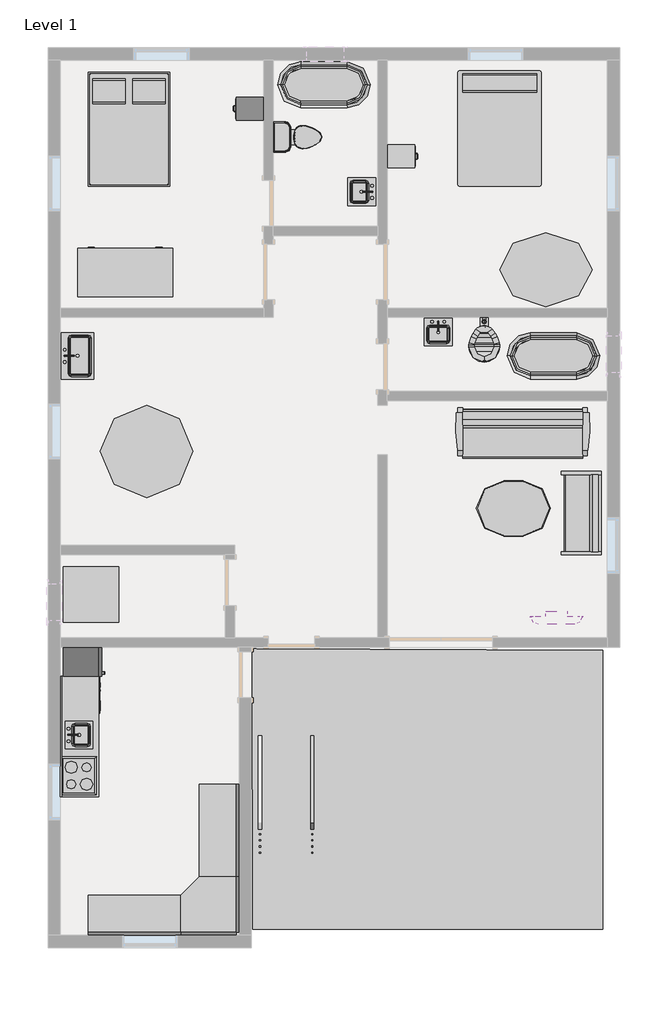
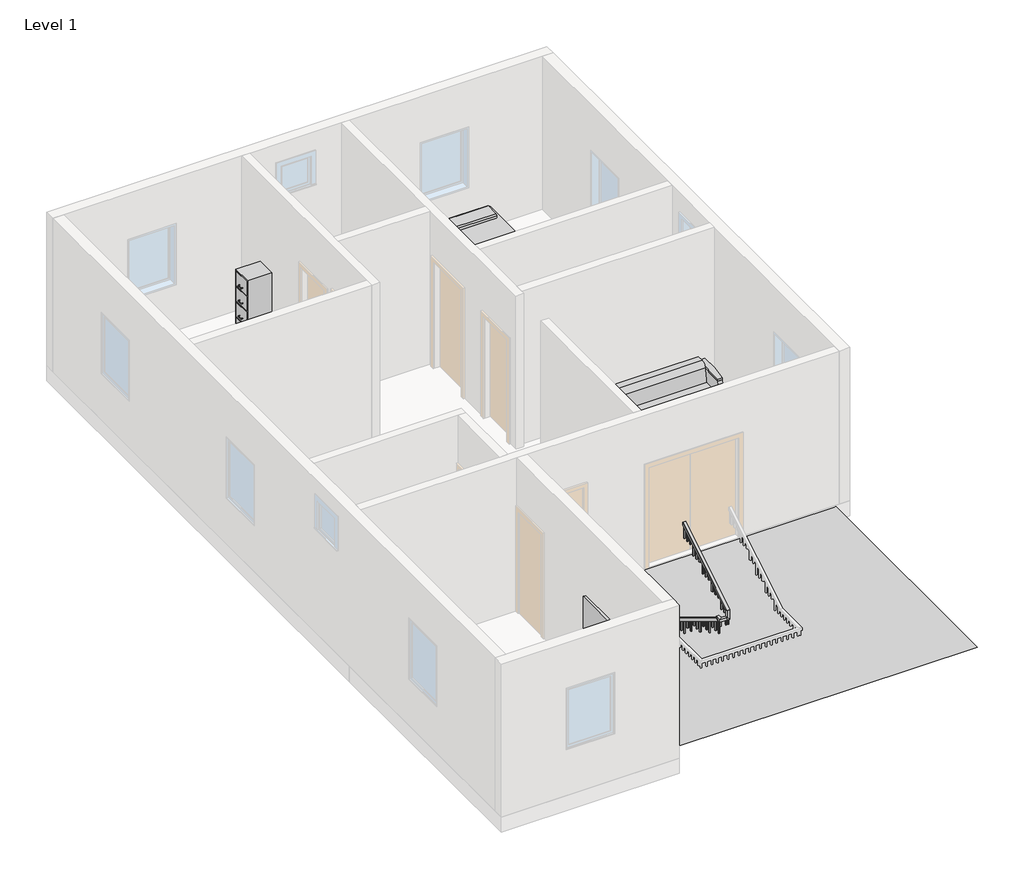
# One storey, part 3 of 3: 14 furniture elements, 8 flow terminals, 5 proxies, 1 railing.
"""IFC4 building model written with IfcOpenShell, lengths in millimetres."""

from ifc_helpers import new_model, si_unit, frame, origin, place, context, project, spatial, polyline, outline, extrude, faceted_brep, triangles, transform, mapped, element, save
from components import proxy_a6faaae8, proxy_45b28599, kitchenette_medium_kitchenette_medium_844211aa, proxy_c523a7b7, flow_terminal_871c2e40, flow_terminal_38af2918, flow_terminal_6d55091a, toilet_domestic_3d_toilet_domestic_3d_f7549cf7, toilet_domestic_3d_toilet_domestic_3d_183bbd19, flow_terminal_b374fae2, furniture_c8abb964, furniture_0253826f, furniture_552c1472, furniture_b1353b55, furniture_c6510c7c, furniture_072f6425, furniture_22419f35, furniture_aff9b2fb, furniture_56245f3a, furniture_be1c6672, furniture_bbcc68ce, furniture_743965d2, furniture_4d44e21c, furniture_45e3acac

model = new_model("IFC4")

# Units and contexts
model_context = context("Model", 3, world=origin())
ifc_project = project(units=[si_unit("LENGTHUNIT", "METRE", prefix="MILLI")], contexts=[model_context])

# Site, building, storey
site = spatial("IfcSite", under=ifc_project)
building = spatial("IfcBuilding", under=site)
storey = spatial("IfcBuildingStorey", under=building, Name="Level 1", Elevation=0.0)

# Proxies
placement = place(None, origin())
element("IfcBuildingElementProxy", 1, Name="Building Element Proxy", at=placement, inside=storey, context=model_context, shape_type="Tessellation", body=[
    triangles([(-6247.6186523, -1018.4977884, 0.0), (-8484.721637, 857.7549837, 0.0), (-8391.9662521, -3287.8891365, 0.0), (-4409.9113472, 761.847611, 0.0), (-4097.5498901, -3554.4772247, 0.0), (-4097.5498901, 908.8842756, 0.0), (-9790.3593842, 942.3358675, 0.0), (-9860.8074097, 1063.1095276, 0.0), (-9878.0656586, 1050.5097879, 0.0), (-4097.5498901, 1043.6765568, 0.0), (-9851.9730652, -3554.4772247, 0.0), (-9869.704541, -3554.4772247, 0.0)], [[7, 12, 11], [4, 10, 2], [3, 7, 11], [2, 7, 3], [9, 7, 8], [7, 9, 12], [8, 7, 2], [2, 10, 8], [3, 5, 1], [5, 3, 11], [1, 5, 4], [3, 1, 2], [4, 6, 10], [6, 4, 5], [1, 4, 2]], closed=False),
])
proxy_shape = proxy_a6faaae8(model_context)
element("IfcBuildingElementProxy", 2, Name="Cook Top-4 Unit2 : 22\" x 20\"", ObjectType="Cook Top-4 Unit2 : 22\" x 20\"", at=placement, inside=storey, context=model_context, shape_type="MappedRepresentation", body=[
    mapped(proxy_shape, transform((-12733.5499219, -1027.1773463, 0.0), x_axis=(0.0, 1.0000000000000002, 0.0), y_axis=(-1.0000000000000002, 0.0, 0.0), z_axis=(0.0, 0.0, 1.0))),
])
proxy_2_shape = proxy_45b28599(model_context)
element("IfcBuildingElementProxy", 3, Name="Dishwasher : 24\" x 24\" x 34\"", ObjectType="Dishwasher : 24\" x 24\" x 34\"", at=placement, inside=storey, context=model_context, shape_type="MappedRepresentation", body=[
    mapped(proxy_2_shape, transform((-12441.7003571, -75.9948148, 0.0), x_axis=(0.0, 1.0000000000000002, 0.0), y_axis=(-1.0000000000000002, 0.0, 0.0), z_axis=(0.0, 0.0, 1.0))),
])
kitchenette_medium_kitchenette_medium_shape = kitchenette_medium_kitchenette_medium_844211aa(model_context)
element("IfcBuildingElementProxy", 4, Name="Kitchenette - Medium : Kitchenette - Medium", ObjectType="Kitchenette - Medium : Kitchenette - Medium", at=placement, inside=storey, context=model_context, shape_type="MappedRepresentation", body=[
    mapped(kitchenette_medium_kitchenette_medium_shape, transform((-13038.3499219, -703.0150512, 0.0), x_axis=(0.0, 1.0000000000000002, 0.0), y_axis=(-1.0000000000000002, 0.0, 0.0), z_axis=(0.0, 0.0, 1.0))),
])
proxy_3_shape = proxy_c523a7b7(model_context)
element("IfcBuildingElementProxy", 5, Name="Refrigerator : 24\" x 25\" LH", ObjectType="Refrigerator : 24\" x 25\" LH", at=placement, inside=storey, context=model_context, shape_type="MappedRepresentation", body=[
    mapped(proxy_3_shape, transform((-12687.9009504, 909.5726537, 0.0), x_axis=(0.0, 1.0000000000000002, 0.0), y_axis=(-1.0000000000000002, 0.0, 0.0), z_axis=(0.0, 0.0, 1.0))),
])

# Flow terminals
flow_terminal_shape = flow_terminal_871c2e40(model_context)
element("IfcFlowTerminal", 6, ObjectType="Sink Kitchen-Island : 18\" x 18\"", at=placement, inside=storey, context=model_context, shape_type="MappedRepresentation", body=[
    mapped(flow_terminal_shape, transform((-6826.0877684, 6285.6772526, 0.0), x_axis=(1.0000000000000002, 0.0, 0.0), y_axis=(0.0, 1.0000000000000002, 0.0), z_axis=(0.0, 0.0, 1.0))),
])
element("IfcFlowTerminal", 7, ObjectType="Sink Kitchen-Island : 18\" x 18\"", at=placement, inside=storey, context=model_context, shape_type="MappedRepresentation", body=[
    mapped(flow_terminal_shape, transform((-8074.995323, 8615.1118943, 0.0), x_axis=(0.0, -1.0000000000000007, 0.0), y_axis=(1.0000000000000007, 0.0, 0.0), z_axis=(0.0, 0.0, 1.0))),
])
element("IfcFlowTerminal", 8, ObjectType="Sink Kitchen-Island : 18\" x 18\"", at=placement, inside=storey, context=model_context, shape_type="MappedRepresentation", body=[
    mapped(flow_terminal_shape, transform((-12731.2045208, -369.7665868, -14.4), x_axis=(0.0, 1.0000000000000002, 0.0), y_axis=(-1.0000000000000002, 0.0, 0.0), z_axis=(0.0, 0.0, 1.0))),
])
flow_terminal_2_shape = flow_terminal_38af2918(model_context)
element("IfcFlowTerminal", 9, ObjectType="Sink Kitchen-Single : 30\" x 21\"", at=placement, inside=storey, context=model_context, shape_type="MappedRepresentation", body=[
    mapped(flow_terminal_2_shape, transform((-12756.6045208, 5878.6334132, 0.0), x_axis=(0.0, 1.0000000000000002, 0.0), y_axis=(-1.0000000000000002, 0.0, 0.0), z_axis=(0.0, 0.0, 1.0))),
])
flow_terminal_3_shape = flow_terminal_6d55091a(model_context)
element("IfcFlowTerminal", 10, ObjectType="Toilet-Commercial-Wall-3D : 15\" Seat Height", at=placement, inside=storey, context=model_context, shape_type="MappedRepresentation", body=[
    mapped(flow_terminal_3_shape, transform((-5648.4467681, 6605.5226537, 0.0), x_axis=(-1.0, 0.0, 0.0), y_axis=(0.0, -1.0, 0.0), z_axis=(0.0, 0.0, 1.0))),
])
toilet_domestic_3d_toilet_domestic_3d_shape = toilet_domestic_3d_toilet_domestic_3d_f7549cf7(model_context)
toilet_domestic_3d_toilet_domestic_3d_2_shape = toilet_domestic_3d_toilet_domestic_3d_183bbd19(model_context)
element("IfcFlowTerminal", 11, ObjectType="Toilet-Domestic-3D : Toilet-Domestic-3D", at=placement, inside=storey, context=model_context, shape_type="MappedRepresentation", body=[
    mapped(toilet_domestic_3d_toilet_domestic_3d_shape, transform((-9038.4538946, 9501.1226537, 0.0), x_axis=(0.0, 1.0, 0.0), y_axis=(-1.0, 0.0, 0.0), z_axis=(0.0, 0.0, 1.0))),
    mapped(toilet_domestic_3d_toilet_domestic_3d_2_shape, transform((-9038.4538946, 9501.1226537, 0.0), x_axis=(0.0, 1.0, 0.0), y_axis=(-1.0, 0.0, 0.0), z_axis=(0.0, 0.0, 1.0))),
])
flow_terminal_4_shape = flow_terminal_b374fae2(model_context)
element("IfcFlowTerminal", 12, ObjectType="Tub-Free Standing-3D : 30\" x 60\"", at=placement, inside=storey, context=model_context, shape_type="MappedRepresentation", body=[
    mapped(flow_terminal_4_shape, transform((-4910.3499219, 5894.3226537, 0.0), x_axis=(0.0, -0.9999999999999998, 0.0), y_axis=(0.9999999999999998, 0.0, 0.0), z_axis=(0.0, 0.0, 1.0))),
])
element("IfcFlowTerminal", 13, ObjectType="Tub-Free Standing-3D : 30\" x 60\"", at=placement, inside=storey, context=model_context, shape_type="MappedRepresentation", body=[
    mapped(flow_terminal_4_shape, transform((-8694.9499219, 10364.7226537, 0.0), x_axis=(0.0, 1.0000000000000002, 0.0), y_axis=(-1.0000000000000002, 0.0, 0.0), z_axis=(0.0, 0.0, 1.0))),
])

# Furniture
furniture_shape = furniture_c8abb964(model_context)
element("IfcFurniture", 14, ObjectType="Bed-Box : Double 53\" x 74\"", at=placement, inside=storey, context=model_context, shape_type="MappedRepresentation", body=[
    mapped(furniture_shape, transform((-12247.2023809, 9862.5521619, 0.0), x_axis=(1.0, 0.0, 0.0), y_axis=(0.0, 1.0, 0.0), z_axis=(0.0, 0.0, 1.0))),
])
furniture_2_shape = furniture_0253826f(model_context)
element("IfcFurniture", 15, ObjectType="Bed-Standard : Double 54\" x 75\"", at=placement, inside=storey, context=model_context, shape_type="MappedRepresentation", body=[
    mapped(furniture_2_shape, transform((-6070.8384465, 9686.4177357, 0.0), x_axis=(1.0, 0.0, 0.0), y_axis=(0.0, 1.0, 0.0), z_axis=(0.0, 0.0, 1.0))),
])
furniture_3_shape = furniture_552c1472(model_context)
element("IfcFurniture", 16, ObjectType="Cabinet-File 3 Drawer : 15\" x 18\"", at=placement, inside=storey, context=model_context, shape_type="MappedRepresentation", body=[
    mapped(furniture_3_shape, transform((-7567.084222, 9311.5191008, 0.0), x_axis=(0.0, 1.0000000000000002, 0.0), y_axis=(-1.0000000000000002, 0.0, 0.0), z_axis=(0.0, 0.0, 1.0))),
])
furniture_4_shape = furniture_b1353b55(model_context)
element("IfcFurniture", 17, ObjectType="Cabinet-File 4 Drawer : 15\" x 18\"", at=placement, inside=storey, context=model_context, shape_type="MappedRepresentation", body=[
    mapped(furniture_4_shape, transform((-9772.0156218, 9843.1262067, 0.0), x_axis=(0.0, -1.0000000000000004, 0.0), y_axis=(1.0000000000000004, 0.0, 0.0), z_axis=(0.0, 0.0, 1.0))),
])
furniture_5_shape = furniture_c6510c7c(model_context)
element("IfcFurniture", 18, ObjectType="Counter Top w Sink Hole : 24\" Depth", at=placement, inside=storey, context=model_context, shape_type="MappedRepresentation", body=[
    mapped(furniture_5_shape, transform((-13038.3499219, -169.6150512, -14.4), x_axis=(0.0, 1.0000000000000002, 0.0), y_axis=(-1.0000000000000002, 0.0, 0.0), z_axis=(0.0, 0.0, 1.0))),
])
furniture_6_shape = furniture_072f6425(model_context)
element("IfcFurniture", 19, ObjectType="Desk : 60\" x 30\"", at=placement, inside=storey, context=model_context, shape_type="MappedRepresentation", body=[
    mapped(furniture_6_shape, transform((-12733.5499219, 6884.9226537, 0.0), x_axis=(1.0, 0.0, 0.0), y_axis=(0.0, 1.0, 0.0), z_axis=(0.0, 0.0, 1.0))),
])
furniture_7_shape = furniture_22419f35(model_context)
element("IfcFurniture", 20, ObjectType="Sofa : 54\"", at=placement, inside=storey, context=model_context, shape_type="MappedRepresentation", body=[
    mapped(furniture_7_shape, transform((-4599.3040203, 3373.8931455, 0.0), x_axis=(0.0, -1.0000000000000004, 0.0), y_axis=(1.0000000000000004, 0.0, 0.0), z_axis=(0.0, 0.0, 1.0))),
])
furniture_8_shape = furniture_aff9b2fb(model_context)
element("IfcFurniture", 21, ObjectType="Sofa-Pensi : 84\"", at=placement, inside=storey, context=model_context, shape_type="MappedRepresentation", body=[
    mapped(furniture_8_shape, transform((-5696.9561719, 4347.2128177, 0.0), x_axis=(1.0, 0.0, 0.0), y_axis=(0.0, 1.0, 0.0), z_axis=(0.0, 0.0, 1.0))),
])
furniture_9_shape = furniture_56245f3a(model_context)
element("IfcFurniture", 22, ObjectType="TV - Flat Screen : 32\"", at=placement, inside=storey, context=model_context, shape_type="MappedRepresentation", body=[
    mapped(furniture_9_shape, transform((-4863.4944361, 1532.230645, 1219.2), x_axis=(-1.0000000000000004, 0.0, 0.0), y_axis=(0.0, -1.0000000000000004, 0.0), z_axis=(0.0, 0.0, 1.0))),
])
furniture_10_shape = furniture_be1c6672(model_context)
element("IfcFurniture", 23, ObjectType="Table-Dining Oval : 36\" x 48\"", at=placement, inside=storey, context=model_context, shape_type="MappedRepresentation", body=[
    mapped(furniture_10_shape, transform((-5168.9302498, 3737.8210144, 0.0), x_axis=(1.0, 0.0, 0.0), y_axis=(0.0, 1.0, 0.0), z_axis=(0.0, 0.0, 1.0))),
])
furniture_11_shape = furniture_bbcc68ce(model_context)
element("IfcFurniture", 24, ObjectType="Table-Dining Round w Chairs : 60\" Diameter", at=placement, inside=storey, context=model_context, shape_type="MappedRepresentation", body=[
    mapped(furniture_11_shape, transform((-11719.6318891, 4504.4013423, 0.0), x_axis=(1.0, 0.0, 0.0), y_axis=(0.0, 1.0, 0.0), z_axis=(0.0, 0.0, 1.0))),
])
furniture_12_shape = furniture_743965d2(model_context)
element("IfcFurniture", 25, ObjectType="Table-Ellipse : 60\" x 48\"", at=placement, inside=storey, context=model_context, shape_type="MappedRepresentation", body=[
    mapped(furniture_12_shape, transform((-5037.3499219, 7316.7226537, 0.0), x_axis=(1.0, 0.0, 0.0), y_axis=(0.0, 1.0, 0.0), z_axis=(0.0, 0.0, 1.0))),
])
furniture_13_shape = furniture_4d44e21c(model_context)
element("IfcFurniture", 26, ObjectType="Table-Rectangular : 36\" x 36\"", at=placement, inside=storey, context=model_context, shape_type="MappedRepresentation", body=[
    mapped(furniture_13_shape, transform((-12530.3499219, 1957.3226537, 0.0), x_axis=(1.0, 0.0, 0.0), y_axis=(0.0, 1.0, 0.0), z_axis=(0.0, 0.0, 1.0))),
])
furniture_14_shape = furniture_45e3acac(model_context)
element("IfcFurniture", 27, ObjectType="Work Station Cubicle : 96\" x 96\"", at=placement, inside=storey, context=model_context, shape_type="MappedRepresentation", body=[
    mapped(furniture_14_shape, transform((-10223.6816741, -4151.1003539, 0.0), x_axis=(-1.0000000000000002, 0.0, 0.0), y_axis=(0.0, -1.0000000000000002, 0.0), z_axis=(0.0, 0.0, 1.0))),
])

# Railing
element("IfcRailing", 28, ObjectType="Handrail - Rectangular", at=placement, inside=storey, context=model_context, shape_type="SolidModel", body=[
    faceted_brep([(-8859.0101729, -363.6715372, 321.7333333), (-8859.0101729, -363.6715372, 262.3318731), (-8909.8101729, -363.6715372, 262.3318731), (-8909.8101729, -363.6715372, 321.7333333), (-8859.0101729, -3360.8715372, 2138.2181818), (-8859.0101729, -3411.6715372, 2109.6046004), (-8909.8101729, -3411.6715372, 2109.6046004), (-8909.8101729, -3360.8715372, 2138.2181818), (-8859.0101729, -3360.8715372, 2184.4), (-8859.0101729, -3411.6715372, 2133.6), (-8909.8101729, -3411.6715372, 2133.6), (-8909.8101729, -3360.8715372, 2184.4), (-8859.0101729, -3437.0715372, 2184.4), (-8859.0101729, -3437.0715372, 2133.6), (-8909.8101729, -3487.8715372, 2133.6), (-8909.8101729, -3487.8715372, 2184.4), (-8782.8101729, -3437.0715372, 2184.4), (-8782.8101729, -3437.0715372, 2133.6), (-8782.8101729, -3487.8715372, 2133.6), (-8782.8101729, -3487.8715372, 2184.4), (-8771.8798033, -3437.0715372, 2184.4), (-8771.8798033, -3487.8715372, 2184.4), (-8721.0798033, -3487.8715372, 2133.6), (-8721.0798033, -3437.0715372, 2133.6)], [[[0, 1, 2, 3]], [[1, 0, 4, 5]], [[2, 1, 5, 6]], [[3, 2, 6, 7]], [[0, 3, 7, 4]], [[5, 4, 8, 9]], [[6, 5, 9, 10]], [[7, 6, 10, 11]], [[4, 7, 11, 8]], [[9, 8, 12, 13]], [[10, 9, 13, 14]], [[11, 10, 14, 15]], [[8, 11, 15, 12]], [[13, 12, 16, 17]], [[14, 13, 17, 18]], [[15, 14, 18, 19]], [[12, 15, 19, 16]], [[20, 21, 22, 23]], [[17, 16, 20, 23]], [[18, 17, 23, 22]], [[19, 18, 22, 21]], [[16, 19, 21, 20]]]),
    faceted_brep([(-8771.8798033, -3437.0715372, 2184.4), (-8721.0798033, -3437.0715372, 2133.6), (-8721.0798033, -3487.8715372, 2133.6), (-8771.8798033, -3487.8715372, 2184.4), (-8771.8798033, -3437.0715372, 2294.3318731), (-8771.8798033, -3487.8715372, 2322.9454545), (-8721.0798033, -3487.8715372, 2322.9454545), (-8721.0798033, -3437.0715372, 2294.3318731)], [[[0, 1, 2, 3]], [[4, 5, 6, 7]], [[1, 0, 4, 7]], [[2, 1, 7, 6]], [[3, 2, 6, 5]], [[0, 3, 5, 4]]]),
    faceted_brep([(-8771.8798033, -3487.8715372, 2322.9454545), (-8771.8798033, -3437.0715372, 2294.3318731), (-8721.0798033, -3437.0715372, 2294.3318731), (-8721.0798033, -3487.8715372, 2322.9454545), (-8771.8798033, -2040.0715372, 3200.4), (-8721.0798033, -2040.0715372, 3200.4), (-8721.0798033, -2040.0715372, 3140.9985397), (-8771.8798033, -2040.0715372, 3140.9985397)], [[[0, 1, 2, 3]], [[4, 5, 6, 7]], [[1, 0, 4, 7]], [[2, 1, 7, 6]], [[3, 2, 6, 5]], [[0, 3, 5, 4]]]),
    extrude(outline(polyline([(-2132.1465372, 3085.1955094), (-2132.1465372, 2878.6666667), (-2151.1965372, 2878.6666667), (-2151.1965372, 3073.6500549), (-2132.1465372, 3085.1955094)])), frame((-8756.0048033, 0.0, 0.0), z_axis=(1.0, 0.0, 0.0), x_axis=(0.0, 1.0, 0.0)), (0.0, 0.0, 1.0), 19.05),
    extrude(outline(polyline([(-2233.7465372, 3023.6197519), (-2233.7465372, 2878.6666667), (-2252.7965372, 2878.6666667), (-2252.7965372, 3012.0742973), (-2233.7465372, 3023.6197519)])), frame((-8756.0048033, 0.0, 0.0), z_axis=(1.0, 0.0, 0.0), x_axis=(0.0, 1.0, 0.0)), (0.0, 0.0, 1.0), 19.05),
    extrude(outline(polyline([(-2335.3465372, 2962.0439943), (-2335.3465372, 2709.3333333), (-2354.3965372, 2709.3333333), (-2354.3965372, 2950.4985397), (-2335.3465372, 2962.0439943)])), frame((-8756.0048033, 0.0, 0.0), z_axis=(1.0, 0.0, 0.0), x_axis=(0.0, 1.0, 0.0)), (0.0, 0.0, 1.0), 19.05),
    extrude(outline(polyline([(-2436.9465372, 2900.4682367), (-2436.9465372, 2709.3333333), (-2455.9965372, 2709.3333333), (-2455.9965372, 2888.9227822), (-2436.9465372, 2900.4682367)])), frame((-8756.0048033, 0.0, 0.0), z_axis=(1.0, 0.0, 0.0), x_axis=(0.0, 1.0, 0.0)), (0.0, 0.0, 1.0), 19.05),
    extrude(outline(polyline([(-2538.5465372, 2838.8924791), (-2538.5465372, 2709.3333333), (-2557.5965372, 2709.3333333), (-2557.5965372, 2827.3470246), (-2538.5465372, 2838.8924791)])), frame((-8756.0048033, 0.0, 0.0), z_axis=(1.0, 0.0, 0.0), x_axis=(0.0, 1.0, 0.0)), (0.0, 0.0, 1.0), 19.05),
    extrude(outline(polyline([(-2640.1465372, 2777.3167216), (-2640.1465372, 2540.0), (-2659.1965372, 2540.0), (-2659.1965372, 2765.771267), (-2640.1465372, 2777.3167216)])), frame((-8756.0048033, 0.0, 0.0), z_axis=(1.0, 0.0, 0.0), x_axis=(0.0, 1.0, 0.0)), (0.0, 0.0, 1.0), 19.05),
    extrude(outline(polyline([(-2741.7465372, 2715.740964), (-2741.7465372, 2540.0), (-2760.7965372, 2540.0), (-2760.7965372, 2704.1955094), (-2741.7465372, 2715.740964)])), frame((-8756.0048033, 0.0, 0.0), z_axis=(1.0, 0.0, 0.0), x_axis=(0.0, 1.0, 0.0)), (0.0, 0.0, 1.0), 19.05),
    extrude(outline(polyline([(-2843.3465372, 2654.1652064), (-2843.3465372, 2540.0), (-2862.3965372, 2540.0), (-2862.3965372, 2642.6197519), (-2843.3465372, 2654.1652064)])), frame((-8756.0048033, 0.0, 0.0), z_axis=(1.0, 0.0, 0.0), x_axis=(0.0, 1.0, 0.0)), (0.0, 0.0, 1.0), 19.05),
    extrude(outline(polyline([(-2944.9465372, 2592.5894488), (-2944.9465372, 2370.6666667), (-2963.9965372, 2370.6666667), (-2963.9965372, 2581.0439943), (-2944.9465372, 2592.5894488)])), frame((-8756.0048033, 0.0, 0.0), z_axis=(1.0, 0.0, 0.0), x_axis=(0.0, 1.0, 0.0)), (0.0, 0.0, 1.0), 19.05),
    extrude(outline(polyline([(-3046.5465372, 2531.0136913), (-3046.5465372, 2370.6666667), (-3065.5965372, 2370.6666667), (-3065.5965372, 2519.4682367), (-3046.5465372, 2531.0136913)])), frame((-8756.0048033, 0.0, 0.0), z_axis=(1.0, 0.0, 0.0), x_axis=(0.0, 1.0, 0.0)), (0.0, 0.0, 1.0), 19.05),
    extrude(outline(polyline([(-3148.1465372, 2469.4379337), (-3148.1465372, 2370.6666667), (-3167.1965372, 2370.6666667), (-3167.1965372, 2457.8924791), (-3148.1465372, 2469.4379337)])), frame((-8756.0048033, 0.0, 0.0), z_axis=(1.0, 0.0, 0.0), x_axis=(0.0, 1.0, 0.0)), (0.0, 0.0, 1.0), 19.05),
    extrude(outline(polyline([(-3249.7465372, 2407.8621761), (-3249.7465372, 2201.3333333), (-3268.7965372, 2201.3333333), (-3268.7965372, 2396.3167216), (-3249.7465372, 2407.8621761)])), frame((-8756.0048033, 0.0, 0.0), z_axis=(1.0, 0.0, 0.0), x_axis=(0.0, 1.0, 0.0)), (0.0, 0.0, 1.0), 19.05),
    extrude(outline(polyline([(-3351.3465372, 2346.2864185), (-3351.3465372, 2201.3333333), (-3370.3965372, 2201.3333333), (-3370.3965372, 2334.740964), (-3351.3465372, 2346.2864185)])), frame((-8756.0048033, 0.0, 0.0), z_axis=(1.0, 0.0, 0.0), x_axis=(0.0, 1.0, 0.0)), (0.0, 0.0, 1.0), 19.05),
    extrude(outline(polyline([(-8792.3351729, -3452.9465372), (-8773.2851729, -3452.9465372), (-8773.2851729, -3471.9965372), (-8792.3351729, -3471.9965372), (-8792.3351729, -3452.9465372)])), frame((0.0, 0.0, 2032.0), z_axis=(0.0, 0.0, 1.0), x_axis=(1.0, 0.0, 0.0)), (0.0, 0.0, 1.0), 101.6),
    extrude(outline(polyline([(-3402.1465372, 2103.8318731), (-3402.1465372, 1862.6666667), (-3421.1965372, 1862.6666667), (-3421.1965372, 2115.3773276), (-3402.1465372, 2103.8318731)])), frame((-8893.9351729, 0.0, 0.0), z_axis=(1.0, 0.0, 0.0), x_axis=(0.0, 1.0, 0.0)), (0.0, 0.0, 1.0), 19.05),
    extrude(outline(polyline([(-3300.5465372, 2042.2561155), (-3300.5465372, 1862.6666667), (-3319.5965372, 1862.6666667), (-3319.5965372, 2053.80157), (-3300.5465372, 2042.2561155)])), frame((-8893.9351729, 0.0, 0.0), z_axis=(1.0, 0.0, 0.0), x_axis=(0.0, 1.0, 0.0)), (0.0, 0.0, 1.0), 19.05),
    extrude(outline(polyline([(-3198.9465372, 1980.6803579), (-3198.9465372, 1862.6666667), (-3217.9965372, 1862.6666667), (-3217.9965372, 1992.2258125), (-3198.9465372, 1980.6803579)])), frame((-8893.9351729, 0.0, 0.0), z_axis=(1.0, 0.0, 0.0), x_axis=(0.0, 1.0, 0.0)), (0.0, 0.0, 1.0), 19.05),
    extrude(outline(polyline([(-3097.3465372, 1919.1046004), (-3097.3465372, 1693.3333333), (-3116.3965372, 1693.3333333), (-3116.3965372, 1930.6500549), (-3097.3465372, 1919.1046004)])), frame((-8893.9351729, 0.0, 0.0), z_axis=(1.0, 0.0, 0.0), x_axis=(0.0, 1.0, 0.0)), (0.0, 0.0, 1.0), 19.05),
    extrude(outline(polyline([(-2995.7465372, 1857.5288428), (-2995.7465372, 1693.3333333), (-3014.7965372, 1693.3333333), (-3014.7965372, 1869.0742973), (-2995.7465372, 1857.5288428)])), frame((-8893.9351729, 0.0, 0.0), z_axis=(1.0, 0.0, 0.0), x_axis=(0.0, 1.0, 0.0)), (0.0, 0.0, 1.0), 19.05),
    extrude(outline(polyline([(-2894.1465372, 1795.9530852), (-2894.1465372, 1693.3333333), (-2913.1965372, 1693.3333333), (-2913.1965372, 1807.4985397), (-2894.1465372, 1795.9530852)])), frame((-8893.9351729, 0.0, 0.0), z_axis=(1.0, 0.0, 0.0), x_axis=(0.0, 1.0, 0.0)), (0.0, 0.0, 1.0), 19.05),
    extrude(outline(polyline([(-2792.5465372, 1734.3773276), (-2792.5465372, 1524.0), (-2811.5965372, 1524.0), (-2811.5965372, 1745.9227822), (-2792.5465372, 1734.3773276)])), frame((-8893.9351729, 0.0, 0.0), z_axis=(1.0, 0.0, 0.0), x_axis=(0.0, 1.0, 0.0)), (0.0, 0.0, 1.0), 19.05),
    extrude(outline(polyline([(-2690.9465372, 1672.80157), (-2690.9465372, 1524.0), (-2709.9965372, 1524.0), (-2709.9965372, 1684.3470246), (-2690.9465372, 1672.80157)])), frame((-8893.9351729, 0.0, 0.0), z_axis=(1.0, 0.0, 0.0), x_axis=(0.0, 1.0, 0.0)), (0.0, 0.0, 1.0), 19.05),
    extrude(outline(polyline([(-2589.3465372, 1611.2258125), (-2589.3465372, 1524.0), (-2608.3965372, 1524.0), (-2608.3965372, 1622.771267), (-2589.3465372, 1611.2258125)])), frame((-8893.9351729, 0.0, 0.0), z_axis=(1.0, 0.0, 0.0), x_axis=(0.0, 1.0, 0.0)), (0.0, 0.0, 1.0), 19.05),
    extrude(outline(polyline([(-2487.7465372, 1549.6500549), (-2487.7465372, 1354.6666667), (-2506.7965372, 1354.6666667), (-2506.7965372, 1561.1955094), (-2487.7465372, 1549.6500549)])), frame((-8893.9351729, 0.0, 0.0), z_axis=(1.0, 0.0, 0.0), x_axis=(0.0, 1.0, 0.0)), (0.0, 0.0, 1.0), 19.05),
    extrude(outline(polyline([(-2386.1465372, 1488.0742973), (-2386.1465372, 1354.6666667), (-2405.1965372, 1354.6666667), (-2405.1965372, 1499.6197519), (-2386.1465372, 1488.0742973)])), frame((-8893.9351729, 0.0, 0.0), z_axis=(1.0, 0.0, 0.0), x_axis=(0.0, 1.0, 0.0)), (0.0, 0.0, 1.0), 19.05),
    extrude(outline(polyline([(-2284.5465372, 1426.4985397), (-2284.5465372, 1185.3333333), (-2303.5965372, 1185.3333333), (-2303.5965372, 1438.0439943), (-2284.5465372, 1426.4985397)])), frame((-8893.9351729, 0.0, 0.0), z_axis=(1.0, 0.0, 0.0), x_axis=(0.0, 1.0, 0.0)), (0.0, 0.0, 1.0), 19.05),
    extrude(outline(polyline([(-2182.9465372, 1364.9227822), (-2182.9465372, 1185.3333333), (-2201.9965372, 1185.3333333), (-2201.9965372, 1376.4682367), (-2182.9465372, 1364.9227822)])), frame((-8893.9351729, 0.0, 0.0), z_axis=(1.0, 0.0, 0.0), x_axis=(0.0, 1.0, 0.0)), (0.0, 0.0, 1.0), 19.05),
    extrude(outline(polyline([(-2081.3465372, 1303.3470246), (-2081.3465372, 1185.3333333), (-2100.3965372, 1185.3333333), (-2100.3965372, 1314.8924791), (-2081.3465372, 1303.3470246)])), frame((-8893.9351729, 0.0, 0.0), z_axis=(1.0, 0.0, 0.0), x_axis=(0.0, 1.0, 0.0)), (0.0, 0.0, 1.0), 19.05),
    extrude(outline(polyline([(-1979.7465372, 1241.771267), (-1979.7465372, 1016.0), (-1998.7965372, 1016.0), (-1998.7965372, 1253.3167216), (-1979.7465372, 1241.771267)])), frame((-8893.9351729, 0.0, 0.0), z_axis=(1.0, 0.0, 0.0), x_axis=(0.0, 1.0, 0.0)), (0.0, 0.0, 1.0), 19.05),
    extrude(outline(polyline([(-1878.1465372, 1180.1955094), (-1878.1465372, 1016.0), (-1897.1965372, 1016.0), (-1897.1965372, 1191.740964), (-1878.1465372, 1180.1955094)])), frame((-8893.9351729, 0.0, 0.0), z_axis=(1.0, 0.0, 0.0), x_axis=(0.0, 1.0, 0.0)), (0.0, 0.0, 1.0), 19.05),
    extrude(outline(polyline([(-1776.5465372, 1118.6197519), (-1776.5465372, 1016.0), (-1795.5965372, 1016.0), (-1795.5965372, 1130.1652064), (-1776.5465372, 1118.6197519)])), frame((-8893.9351729, 0.0, 0.0), z_axis=(1.0, 0.0, 0.0), x_axis=(0.0, 1.0, 0.0)), (0.0, 0.0, 1.0), 19.05),
    extrude(outline(polyline([(-1674.9465372, 1057.0439943), (-1674.9465372, 846.6666667), (-1693.9965372, 846.6666667), (-1693.9965372, 1068.5894488), (-1674.9465372, 1057.0439943)])), frame((-8893.9351729, 0.0, 0.0), z_axis=(1.0, 0.0, 0.0), x_axis=(0.0, 1.0, 0.0)), (0.0, 0.0, 1.0), 19.05),
    extrude(outline(polyline([(-1573.3465372, 995.4682367), (-1573.3465372, 846.6666667), (-1592.3965372, 846.6666667), (-1592.3965372, 1007.0136913), (-1573.3465372, 995.4682367)])), frame((-8893.9351729, 0.0, 0.0), z_axis=(1.0, 0.0, 0.0), x_axis=(0.0, 1.0, 0.0)), (0.0, 0.0, 1.0), 19.05),
    extrude(outline(polyline([(-1471.7465372, 933.8924791), (-1471.7465372, 846.6666667), (-1490.7965372, 846.6666667), (-1490.7965372, 945.4379337), (-1471.7465372, 933.8924791)])), frame((-8893.9351729, 0.0, 0.0), z_axis=(1.0, 0.0, 0.0), x_axis=(0.0, 1.0, 0.0)), (0.0, 0.0, 1.0), 19.05),
    extrude(outline(polyline([(-1370.1465372, 872.3167216), (-1370.1465372, 677.3333333), (-1389.1965372, 677.3333333), (-1389.1965372, 883.8621761), (-1370.1465372, 872.3167216)])), frame((-8893.9351729, 0.0, 0.0), z_axis=(1.0, 0.0, 0.0), x_axis=(0.0, 1.0, 0.0)), (0.0, 0.0, 1.0), 19.05),
    extrude(outline(polyline([(-1268.5465372, 810.740964), (-1268.5465372, 677.3333333), (-1287.5965372, 677.3333333), (-1287.5965372, 822.2864185), (-1268.5465372, 810.740964)])), frame((-8893.9351729, 0.0, 0.0), z_axis=(1.0, 0.0, 0.0), x_axis=(0.0, 1.0, 0.0)), (0.0, 0.0, 1.0), 19.05),
    extrude(outline(polyline([(-1166.9465372, 749.1652064), (-1166.9465372, 508.0), (-1185.9965372, 508.0), (-1185.9965372, 760.710661), (-1166.9465372, 749.1652064)])), frame((-8893.9351729, 0.0, 0.0), z_axis=(1.0, 0.0, 0.0), x_axis=(0.0, 1.0, 0.0)), (0.0, 0.0, 1.0), 19.05),
    extrude(outline(polyline([(-1065.3465372, 687.5894488), (-1065.3465372, 508.0), (-1084.3965372, 508.0), (-1084.3965372, 699.1349034), (-1065.3465372, 687.5894488)])), frame((-8893.9351729, 0.0, 0.0), z_axis=(1.0, 0.0, 0.0), x_axis=(0.0, 1.0, 0.0)), (0.0, 0.0, 1.0), 19.05),
    extrude(outline(polyline([(-963.7465372, 626.0136913), (-963.7465372, 508.0), (-982.7965372, 508.0), (-982.7965372, 637.5591458), (-963.7465372, 626.0136913)])), frame((-8893.9351729, 0.0, 0.0), z_axis=(1.0, 0.0, 0.0), x_axis=(0.0, 1.0, 0.0)), (0.0, 0.0, 1.0), 19.05),
    extrude(outline(polyline([(-862.1465372, 564.4379337), (-862.1465372, 338.6666667), (-881.1965372, 338.6666667), (-881.1965372, 575.9833882), (-862.1465372, 564.4379337)])), frame((-8893.9351729, 0.0, 0.0), z_axis=(1.0, 0.0, 0.0), x_axis=(0.0, 1.0, 0.0)), (0.0, 0.0, 1.0), 19.05),
    extrude(outline(polyline([(-760.5465372, 502.8621761), (-760.5465372, 338.6666667), (-779.5965372, 338.6666667), (-779.5965372, 514.4076307), (-760.5465372, 502.8621761)])), frame((-8893.9351729, 0.0, 0.0), z_axis=(1.0, 0.0, 0.0), x_axis=(0.0, 1.0, 0.0)), (0.0, 0.0, 1.0), 19.05),
    extrude(outline(polyline([(-658.9465372, 441.2864185), (-658.9465372, 338.6666667), (-677.9965372, 338.6666667), (-677.9965372, 452.8318731), (-658.9465372, 441.2864185)])), frame((-8893.9351729, 0.0, 0.0), z_axis=(1.0, 0.0, 0.0), x_axis=(0.0, 1.0, 0.0)), (0.0, 0.0, 1.0), 19.05),
    extrude(outline(polyline([(-557.3465372, 379.710661), (-557.3465372, 169.3333333), (-576.3965372, 169.3333333), (-576.3965372, 391.2561155), (-557.3465372, 379.710661)])), frame((-8893.9351729, 0.0, 0.0), z_axis=(1.0, 0.0, 0.0), x_axis=(0.0, 1.0, 0.0)), (0.0, 0.0, 1.0), 19.05),
    extrude(outline(polyline([(-455.7465372, 318.1349034), (-455.7465372, 169.3333333), (-474.7965372, 169.3333333), (-474.7965372, 329.6803579), (-455.7465372, 318.1349034)])), frame((-8893.9351729, 0.0, 0.0), z_axis=(1.0, 0.0, 0.0), x_axis=(0.0, 1.0, 0.0)), (0.0, 0.0, 1.0), 19.05),
    extrude(outline(polyline([(-8756.0048033, -3471.9965372), (-8756.0048033, -3452.9465372), (-8736.9548033, -3452.9465372), (-8736.9548033, -3471.9965372), (-8756.0048033, -3471.9965372)])), frame((0.0, 0.0, 2032.0), z_axis=(0.0, 0.0, 1.0), x_axis=(1.0, 0.0, 0.0)), (0.0, 0.0, 1.0), 104.6787879),
    extrude(outline(polyline([(-8874.8851729, -3452.9465372), (-8874.8851729, -3471.9965372), (-8893.9351729, -3471.9965372), (-8893.9351729, -3452.9465372), (-8874.8851729, -3452.9465372)])), frame((0.0, 0.0, 2032.0), z_axis=(0.0, 0.0, 1.0), x_axis=(1.0, 0.0, 0.0)), (0.0, 0.0, 1.0), 101.6),
    extrude(outline(polyline([(-8874.8851729, -3427.5465372), (-8874.8851729, -3446.5965372), (-8893.9351729, -3446.5965372), (-8893.9351729, -3427.5465372), (-8874.8851729, -3427.5465372)])), frame((0.0, 0.0, 2032.0), z_axis=(0.0, 0.0, 1.0), x_axis=(1.0, 0.0, 0.0)), (0.0, 0.0, 1.0), 101.6),
    extrude(outline(polyline([(-2040.0715372, 3140.9985397), (-2040.0715372, 2878.6666667), (-2059.1215372, 2878.6666667), (-2059.1215372, 3129.4530852), (-2040.0715372, 3140.9985397)])), frame((-8756.0048033, 0.0, 0.0), z_axis=(1.0, 0.0, 0.0), x_axis=(0.0, 1.0, 0.0)), (0.0, 0.0, 1.0), 19.05),
    extrude(outline(polyline([(-363.6715372, 262.3318731), (-363.6715372, 169.3333333), (-382.7215372, 169.3333333), (-382.7215372, 273.8773276), (-363.6715372, 262.3318731)])), frame((-8893.9351729, 0.0, 0.0), z_axis=(1.0, 0.0, 0.0), x_axis=(0.0, 1.0, 0.0)), (0.0, 0.0, 1.0), 19.05),
])

save(model, "model.ifc")

# Revit data of these elements
# Type "Cook Top-4 Unit2 : 22\" x 20\""
#   Depth = 1' - 8"
#   Width = 1' - 10"
#   Burner Material = Steel, Chrome Plated
#   Cooktop Material = Steel, Polished
#   Default Elevation = 0
#   Assembly Code = ""
# Type "Dishwasher : 24\" x 24\" x 34\""
#   Label = "DW"
#   Assembly Code = "E1090400"
#   Depth = 2' - 0"
#   Height = 2' - 10"
#   Width = 2' - 0"
#   Dishwasher Material = Steel, Paint Finish, Ivory, Glossy
#   Panel Face Material = Plastic, Opaque Black
#   Default Elevation = 0
# Type "Kitchenette - Medium : Kitchenette - Medium"
#   Assembly Code = "E1090400"
#   Counter Length = 6' - 6"
#   Cabinet Width = 4' - 6"
#   Cabinet Height = 2' - 10 1/2"
#   Cabinet Depth = 2' - 0"
#   Toe Depth = 0' - 3"
#   Toe Height = 0' - 3 1/2"
#   Cabinet Material = Cabinets
#   Door/Drawer Material = Cabinets
#   Handle Material = Cabinets - Handles
#   Default Elevation = 0
# Type "Refrigerator : 24\" x 25\" LH"
#   Label = "REF."
#   Assembly Code = "E1090400"
#   Depth = 2' - 0 3/4"
#   Handle = 0' - 1 1/2"
#   Height = 5' - 3 1/2"
#   Rear Clearance = 0' - 2"
#   Top Door Height = 1' - 8"
#   Width = 1' - 11 1/2"
#   Material = Steel, Paint Finish, Ivory, Glossy
#   Default Elevation = 0
# Type "Sink Kitchen-Island : 18\" x 18\""
#   Assembly Code = "D2010410"
#   Counter Height = 3' - 0"
#   Depth = 1' - 6"
#   Width = 1' - 6"
#   Faucet Material = Steel, Polished
#   Sink Material = Steel, Polished
#   Default Elevation = 0
# Type "Sink Kitchen-Single : 30\" x 21\""
#   Assembly Code = "D2010410"
#   Counter Height = 3' - 0"
#   Depth = 1' - 9"
#   Width = 2' - 6"
#   Faucet Material = Steel, Polished
#   Sink Material = Steel, Polished
#   Default Elevation = 0
# Type "Toilet-Commercial-Wall-3D : 15\" Seat Height"
#   Assembly Code = "D2010110"
#   Mounting Height = 1' - 3"
#   Piping Material = Steel, Polished
#   Toilet - Bowl Material = Porcelain, Ivory
#   Toilet - Seat Material = Laminate, Ivory, Matte
#   Default Elevation = 0
# Type "Toilet-Domestic-3D : Toilet-Domestic-3D"
#   Assembly Code = "D2010110"
#   Toilet - Bowl/Basin Material = Porcelain, Linen
#   Toilet - Seat Material = Laminate, Linen, Matte
#   Default Elevation = 0
# Type "Tub-Free Standing-3D : 30\" x 60\""
#   Assembly Code = "D2010110"
#   Height = 1' - 6"
#   Length = 5' - 0"
#   Width = 2' - 6"
#   Tub Material = Porcelain, Ivory
#   Default Elevation = 0
# Type "Bed-Box : Double 53\" x 74\""
#   Assembly Code = "E2020200"
#   Length = 6' - 2"
#   Width = 4' - 5"
#   Frame Material = Birch
#   Mattress Material = Linen, White
#   Default Elevation = 0
# Type "Bed-Standard : Double 54\" x 75\""
#   Assembly Code = "E2020200"
#   Length = 6' - 3"
#   Width = 4' - 6"
#   Leg Material = Steel, Chrome Plated
#   Mattress Material = Linen, White
#   Default Elevation = 0
# Type "Cabinet-File 3 Drawer : 15\" x 18\""
#   Assembly Code = "E2020200"
#   Depth = 1' - 6"
#   Height = 3' - 5"
#   Width = 1' - 3"
#   Cabinet Material = Steel, Paint Finish, Ivory, Glossy
#   Handle Material = Steel, Chrome Plated
#   Default Elevation = 0
# Type "Cabinet-File 4 Drawer : 15\" x 18\""
#   Assembly Code = "E2020200"
#   Depth = 1' - 6"
#   Height = 4' - 4"
#   Width = 1' - 3"
#   Cabinet Material = Steel, Paint Finish, Ivory, Glossy
#   Handle Material = Steel, Chrome Plated
#   Default Elevation = 0
# Type "Counter Top w Sink Hole : 24\" Depth"
#   Assembly Code = "C1030400"
#   Counter Thickness = 0' - 1 1/2"
#   Depth = 2' - 1"
#   Height = 3' - 0"
#   Length [instance default] = 8' - 0"
#   Sink Location [instance default] = 2' - 0"
#   Sink Location To Wall [instance default] = 0' - 6"
#   Sink Opening Depth [instance default] = 1' - 3"
#   Sink Opening Width [instance default] = 2' - 3"
#   Counter Top Material = none
#   Default Elevation = 0
# Type "Desk : 60\" x 30\""
#   Assembly Code = "E2020200"
#   Depth = 2' - 6"
#   Height = 2' - 6"
#   Leg Height = 0' - 6"
#   Width = 5' - 0"
#   Body Material = Laminate, Ivory, Matte
#   Handle/Leg Material = Steel, Chrome Plated
#   Top Material = Cherry
#   Default Elevation = 0
# Type "Sofa : 54\""
#   Assembly Code = "E2020200"
#   Width = 4' - 6"
#   Seat Material = none
#   Frame Material = none
#   Default Elevation = 0
# Type "Sofa-Pensi : 84\""
#   Assembly Code = "E2020200"
#   Length = 7' - 0"
#   Frame Material = Cherry
#   Seat Material = Linen, Beige
#   Feet Material = Steel, Chrome Plated
#   Default Elevation = 0
# Type "TV - Flat Screen : 32\""
#   SinAng = 0' - 0.0193"
#   L = 2' - 3.79372"
#   H = 1' - 3.6354"
#   Thickness = 0' - 4.33071"
#   Diagonal = 2' - 7.88976"
#   CosAng = 0' - 0.03431"
#   Stand [instance default] = yes
#   Default Elevation = 0
# Type "Table-Dining Oval : 36\" x 48\""
#   Assembly Code = "E2020200"
#   Length = 4' - 0"
#   Width = 3' - 0"
#   Base Material = Steel, Chrome Plated
#   Top Material = Glass - Clear, Grey
#   Default Elevation = 0
#   Description = (empty or 0)
# Type "Table-Dining Round w Chairs : 60\" Diameter"
#   Assembly Code = "E2020200"
#   Radius = 2' - 6"
#   Diameter = 5' - 0"
#   Height = 2' - 6"
#   Chairs = 6
#   Base Material = Pine
#   Top Material = Laminate, Linen, Matte
#   Default Elevation = 0
# Type "Table-Ellipse : 60\" x 48\""
#   Assembly Code = "E2020200"
#   Half Width = 2' - 0"
#   Half Length = 2' - 6"
#   Height = 2' - 6"
#   Length = 5' - 0"
#   Width = 4' - 0"
#   Base Material = Birch
#   Top Material = Birch
#   Default Elevation = 0
# Type "Table-Rectangular : 36\" x 36\""
#   Assembly Code = "E2020200"
#   Height = 2' - 6"
#   Length = 3' - 0"
#   Width = 3' - 0"
#   Base Material = Birch
#   Top Material = Birch
#   Default Elevation = 0
# Type "Work Station Cubicle : 96\" x 96\""
#   Assembly Code = "E2020"
#   Desktop Height = 2' - 6"
#   Desktop1 Width = 2' - 0"
#   Desktop2 Width = 2' - 0"
#   Panel Height = 5' - 6"
#   Panel1 Length = 5' - 0"
#   Panel2 Length = 5' - 0"
#   Cube Panel Material = Textile - Light Gray
#   Work Top Material = Laminate, Ivory, Matte
#   Default Elevation = 0
# Type "Handrail - Rectangular"
#   Assembly Code = "C2010400"
#   built-in parameter 1008612 = 0.0416667 (stored number, unit not read)
#   built-in parameter 1008611 = 0.0416667 (stored number, unit not read)
#   built-in parameter 1008609 = 0.333333 (stored number, unit not read)
#   built-in parameter 1008604 = 0.166667 (stored number, unit not read)
#   built-in parameter 1008603 = 0.166667 (stored number, unit not read)
#   Railing Height = 0' - 6"
#   built-in parameter 1008630 = 2
#   built-in parameter 1008610 = 2
#   built-in parameter 1008618 = Baluster - Square : 3/4"
# Element 1 (IfcBuildingElementProxy)
#   Material = none
#   Phase Created = New Construction
# Element 2 (IfcBuildingElementProxy, "Cook Top-4 Unit2 : 22\" x 20\"")
#   Phase Created = New Construction
#   Materials on its faces: "Steel, Chrome Plated", "Steel, Polished"
# Element 3 (IfcBuildingElementProxy, "Dishwasher : 24\" x 24\" x 34\"")
#   Phase Created = New Construction
#   Materials on its faces: "Steel, Paint Finish, Ivory, Glossy", "Plastic, Opaque Black"
# Element 4 (IfcBuildingElementProxy, "Kitchenette - Medium : Kitchenette - Medium")
#   Phase Created = New Construction
#   Materials on its faces: "Cabinets", "Cabinets - Handles"
# Element 5 (IfcBuildingElementProxy, "Refrigerator : 24\" x 25\" LH")
#   Phase Created = New Construction
#   Materials on its faces: "Steel, Paint Finish, Ivory, Glossy", "Steel, Chrome Plated"
# Element 6 (IfcFlowTerminal, "Sink Kitchen-Island : 18\" x 18\"")
#   Mark = "6"
#   Phase Created = New Construction
#   Materials on its faces: "Steel, Polished"
# Element 7 (IfcFlowTerminal, "Sink Kitchen-Island : 18\" x 18\"")
#   Mark = "7"
#   Phase Created = New Construction
#   Materials on its faces: "Steel, Polished"
# Element 8 (IfcFlowTerminal, "Sink Kitchen-Island : 18\" x 18\"")
#   Mark = "9"
#   Phase Created = New Construction
#   Materials on its faces: "Steel, Polished"
# Element 9 (IfcFlowTerminal, "Sink Kitchen-Single : 30\" x 21\"")
#   Mark = "10"
#   Phase Created = New Construction
#   Materials on its faces: "Steel, Polished"
# Element 10 (IfcFlowTerminal, "Toilet-Commercial-Wall-3D : 15\" Seat Height")
#   Mark = "4"
#   Phase Created = New Construction
#   Materials on its faces: "Laminate, Ivory, Matte", "Porcelain, Ivory", "Steel, Polished"
# Element 11 (IfcFlowTerminal, "Toilet-Domestic-3D : Toilet-Domestic-3D")
#   Mark = "8"
#   Phase Created = New Construction
#   Materials on its faces: "Porcelain, Linen", "Laminate, Linen, Matte"
# Element 12 (IfcFlowTerminal, "Tub-Free Standing-3D : 30\" x 60\"")
#   Mark = "1"
#   Phase Created = New Construction
#   Materials on its faces: "Porcelain, Ivory"
# Element 13 (IfcFlowTerminal, "Tub-Free Standing-3D : 30\" x 60\"")
#   Mark = "2"
#   Phase Created = New Construction
#   Materials on its faces: "Porcelain, Ivory"
# Element 14 (IfcFurniture, "Bed-Box : Double 53\" x 74\"")
#   Phase Created = New Construction
#   Materials on its faces: "Birch", "Linen, White"
# Element 15 (IfcFurniture, "Bed-Standard : Double 54\" x 75\"")
#   Phase Created = New Construction
#   Materials on its faces: "Linen, White", "Steel, Chrome Plated"
# Element 16 (IfcFurniture, "Cabinet-File 3 Drawer : 15\" x 18\"")
#   Phase Created = New Construction
#   Materials on its faces: "Steel, Chrome Plated", "Steel, Paint Finish, Ivory, Glossy"
# Element 17 (IfcFurniture, "Cabinet-File 4 Drawer : 15\" x 18\"")
#   Phase Created = New Construction
#   Materials on its faces: "Steel, Chrome Plated", "Steel, Paint Finish, Ivory, Glossy"
# Element 18 (IfcFurniture, "Counter Top w Sink Hole : 24\" Depth")
#   Sink Opening Depth = 1' - 2"
#   Sink Location To Wall = 0' - 6"
#   Length = 6' - 6"
#   Sink Location = 3' - 4"
#   Sink Opening Width = 1' - 4"
#   Phase Created = New Construction
#   Materials on its faces: "Counter Top"
# Element 19 (IfcFurniture, "Desk : 60\" x 30\"")
#   Phase Created = New Construction
#   Materials on its faces: "Steel, Chrome Plated", "Laminate, Ivory, Matte", "Cherry"
# Element 20 (IfcFurniture, "Sofa : 54\"")
#   Phase Created = New Construction
#   Materials on its faces: "Cherry"
# Element 21 (IfcFurniture, "Sofa-Pensi : 84\"")
#   Phase Created = New Construction
#   Materials on its faces: "Cherry", "Linen, Beige", "Steel, Chrome Plated"
# Element 22 (IfcFurniture, "TV - Flat Screen : 32\"")
#   Stand = yes
#   Phase Created = New Construction
#   Materials on its faces: "TV - Black", "TV - Glass", "TV - Screen"
# Element 23 (IfcFurniture, "Table-Dining Oval : 36\" x 48\"")
#   Phase Created = New Construction
#   Materials on its faces: "Steel, Chrome Plated", "Glass - Clear, Grey"
# Element 24 (IfcFurniture, "Table-Dining Round w Chairs : 60\" Diameter")
#   Phase Created = New Construction
#   Materials on its faces: "Pine", "Laminate, Linen, Matte"
# Element 25 (IfcFurniture, "Table-Ellipse : 60\" x 48\"")
#   Phase Created = New Construction
#   Materials on its faces: "Birch"
# Element 26 (IfcFurniture, "Table-Rectangular : 36\" x 36\"")
#   Phase Created = New Construction
#   Materials on its faces: "Birch"
# Element 27 (IfcFurniture, "Work Station Cubicle : 96\" x 96\"")
#   Phase Created = New Construction
#   Materials on its faces: "Textile - Light Gray", "Laminate, Ivory, Matte"
# Element 28 (IfcRailing, "Handrail - Rectangular")
#   Phase Created = New Construction
# Materials
#   "Steel, Chrome Plated": class "Metal", colour RGB 17 17 17, transparency 0, Description = "Chromiuim plated steel", Cost = 0
#   "Steel, Polished": class "Metal", colour RGB 57 57 57, transparency 0, Description = "Polished steel", Cost = 0
#   "Steel, Paint Finish, Ivory, Glossy": class "Metal", colour RGB 247 247 239, transparency 0, Description = "Steel, paint finish, ivory, glossy", Cost = 0
#   "Plastic, Opaque Black": class "Plastic", colour RGB 0 0 0, transparency 0.7, Description = "Plastic, generic, opaque black", Cost = 0
#   "Cabinets": colour RGB 249 249 249, transparency 0
#   "Cabinets - Handles": class "Metal", colour RGB 57 57 57, transparency 0
#   "Porcelain, Ivory": class "Ceramic", colour RGB 247 247 239, transparency 0, Description = "Porcelain, ivory", Cost = 0
#   "Laminate, Ivory, Matte": class "Plastic", colour RGB 247 247 239, transparency 0, Description = "Plastic Laminate - Ivory, Matte", Cost = 0
#   "Porcelain, Linen": class "Ceramic", colour RGB 249 239 230, transparency 0, Description = "Porcelain, linen", Cost = 0
#   "Laminate, Linen, Matte": class "Plastic", colour RGB 249 239 230, transparency 0, Description = "Plastic Laminate - Linen, Matte", Cost = 0
#   "Birch": class "Wood", colour RGB 224 178 126, transparency 0, Description = "Betula Alleghaniensis", Cost = 0
#   "Linen, White": class "Textile", colour RGB 247 247 239, transparency 0, Description = "Linen, white", Cost = 0
#   "Cherry": class "Wood", colour RGB 226 177 128, transparency 0, Description = "Prunus Serotina", Cost = 0
#   "Linen, Beige": class "Textile", colour RGB 249 239 230, transparency 0, Description = "Linen, beige", Cost = 0
#   "Glass - Clear, Grey": class "Glass", colour RGB 252 255 255, transparency 0.64
#   "Pine": class "Wood", colour RGB 223 192 134, transparency 0, Description = "Pinus Echinata", Cost = 0
#   "Textile - Light Gray": class "Fabric", colour RGB 204 204 204, transparency 0
#   "Counter Top": class "Wood", colour RGB 226 177 128, transparency 0
#   "TV - Black": colour RGB 49 49 49, transparency 0
#   "TV - Glass": colour RGB 157 157 157, transparency 0.9
#   "TV - Screen": colour RGB 0 0 0, transparency 0
